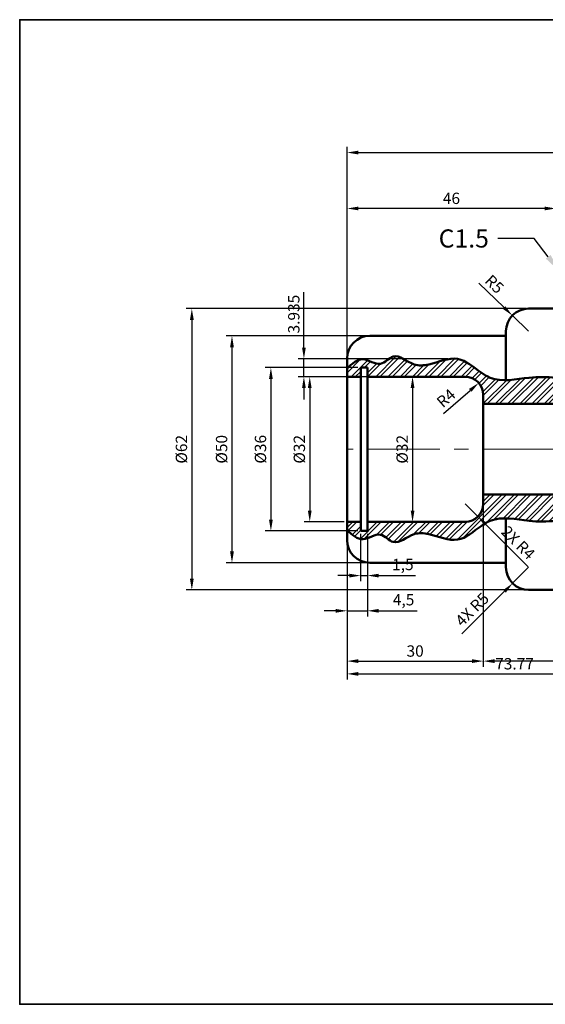
# Model space of a CAD drawing. Units: millimetres. Extents: x 14 to 362, y 30 to 247.
# Tile 1 of 3: x 14 to 130, y 30 to 247. Entities that reach past the tile are written whole.
import ezdxf
from ezdxf import colors
from ezdxf.entities.mleader import LeaderData, LeaderLine
from ezdxf.math import Vec2, Vec3

# ---------------------------------------------------------------- set-up
doc = ezdxf.new("R2010")
doc.units = ezdxf.units.MM
doc.header["$LTSCALE"] = 0.5
doc.linetypes.add('CENTER', pattern=[50.8, 31.75, -6.35, 6.35, -6.35])
for name, color, linetype, lineweight in [('M-CNTR', 1, 'CENTER', 18), ('M-DIMS', 2, 'Continuous', 25), ('M-HATC', 8, 'Continuous', 18), ('M-OUTL', 7, 'Continuous', 50), ('M-TTLB', 7, 'Continuous', 35)]:
    doc.layers.add(name, color=color, linetype=linetype, lineweight=lineweight)
doc.styles.get("Standard").update_dxf_attribs({"font": 'arial.ttf'})
doc.dimstyles.new('ISO-25', dxfattribs={"dimtxt": 2.5, "dimasz": 2.5, "dimexe": 1.25, "dimexo": 0.625, "dimtad": 1, "dimtxsty": 'Standard', "dimcen": 2.5, "dimadec": 0, "dimazin": 0, "dimtfac": 1, "dimtmove": 0, "dimatfit": 3, "dimfxl": 1, "dimarcsym": 0})

# ---------------------------------------------------------------- blocks, each defined once
blk = doc.blocks.new('*D1')
at = {"layer": 'Defpoints', "color": 0, "ltscale": 0.5, "transparency": 16777216}
for p in [(94.08, 177.22), (61.13, 127.22), (94.08, 127.22)]:
    blk.add_point(p, dxfattribs=at)
at = {"layer": 'M-DIMS', "color": 0, "lineweight": -2, "ltscale": 0.5, "transparency": 16777216}
for p, q in [((93.46, 177.22), (59.88, 177.22)), ((61.13, 174.72), (61.13, 129.72)), ((93.46, 127.22), (59.88, 127.22))]:
    blk.add_line(p, q, dxfattribs=at)
at = {"layer": 'M-DIMS', "color": 0, "ltscale": 0.5, "transparency": 16777216}
for points in [[(60.71, 174.72), (61.55, 174.72), (61.13, 177.22)], [(60.71, 129.72), (61.55, 129.72), (61.13, 127.22)]]:
    blk.add_solid(points, dxfattribs=at)
at = {"layer": 'M-DIMS', "color": 0, "ltscale": 0.5, "transparency": 16777216, "insert": (59.16, 152.22), "char_height": 2.5, "attachment_point": 5, "rotation": 90}
blk.add_mtext('%%C50', dxfattribs=at)
blk = doc.blocks.new('*D2')
at = {"layer": 'Defpoints', "color": 0, "ltscale": 0.5, "transparency": 16777216}
for p in [(89.47, 170.22), (69.7, 134.22), (89.47, 134.22)]:
    blk.add_point(p, dxfattribs=at)
at = {"layer": 'M-DIMS', "color": 0, "lineweight": -2, "ltscale": 0.5, "transparency": 16777216}
for p, q in [((88.85, 170.22), (68.45, 170.22)), ((69.7, 167.72), (69.7, 136.72)), ((88.85, 134.22), (68.45, 134.22))]:
    blk.add_line(p, q, dxfattribs=at)
at = {"layer": 'M-DIMS', "color": 0, "ltscale": 0.5, "transparency": 16777216}
for points in [[(69.28, 167.72), (70.12, 167.72), (69.7, 170.22)], [(69.28, 136.72), (70.12, 136.72), (69.7, 134.22)]]:
    blk.add_solid(points, dxfattribs=at)
at = {"layer": 'M-DIMS', "color": 0, "ltscale": 0.5, "transparency": 16777216, "insert": (67.73, 152.22), "char_height": 2.5, "attachment_point": 5, "rotation": 90}
blk.add_mtext('%%C36', dxfattribs=at)
blk = doc.blocks.new('*D3')
at = {"layer": 'Defpoints', "color": 0, "ltscale": 0.5, "transparency": 16777216}
for p in [(86.47, 168.22), (78.26, 136.22), (86.47, 136.22)]:
    blk.add_point(p, dxfattribs=at)
at = {"layer": 'M-DIMS', "color": 0, "lineweight": -2, "ltscale": 0.5, "transparency": 16777216}
for p, q in [((85.85, 168.22), (77.01, 168.22)), ((78.26, 165.72), (78.26, 138.72)), ((85.85, 136.22), (77.01, 136.22))]:
    blk.add_line(p, q, dxfattribs=at)
at = {"layer": 'M-DIMS', "color": 0, "ltscale": 0.5, "transparency": 16777216}
for points in [[(77.84, 165.72), (78.67, 165.72), (78.26, 168.22)], [(77.84, 138.72), (78.67, 138.72), (78.26, 136.22)]]:
    blk.add_solid(points, dxfattribs=at)
at = {"layer": 'M-DIMS', "color": 0, "ltscale": 0.5, "transparency": 16777216, "insert": (76.29, 152.22), "char_height": 2.5, "attachment_point": 5, "rotation": 90}
blk.add_mtext('%%C32', dxfattribs=at)
blk = doc.blocks.new('*D4')
at = {"layer": 'Defpoints', "color": 0, "ltscale": 0.5, "transparency": 16777216}
for p in [(126.47, 183.22), (52.29, 121.22), (126.47, 121.22)]:
    blk.add_point(p, dxfattribs=at)
at = {"layer": 'M-DIMS', "color": 0, "lineweight": -2, "ltscale": 0.5, "transparency": 16777216}
for p, q in [((125.85, 183.22), (51.04, 183.22)), ((52.29, 180.72), (52.29, 123.72)), ((125.85, 121.22), (51.04, 121.22))]:
    blk.add_line(p, q, dxfattribs=at)
at = {"layer": 'M-DIMS', "color": 0, "ltscale": 0.5, "transparency": 16777216}
for points in [[(51.87, 180.72), (52.71, 180.72), (52.29, 183.22)], [(51.87, 123.72), (52.71, 123.72), (52.29, 121.22)]]:
    blk.add_solid(points, dxfattribs=at)
at = {"layer": 'M-DIMS', "color": 0, "ltscale": 0.5, "transparency": 16777216, "insert": (50.32, 152.22), "char_height": 2.5, "attachment_point": 5, "rotation": 90}
blk.add_mtext('%%C62', dxfattribs=at)
blk = doc.blocks.new('*D5')
at = {"layer": 'Defpoints', "color": 0, "ltscale": 0.5, "transparency": 16777216}
for p in [(89.47, 134.22), (90.97, 134.22), (90.97, 124.38)]:
    blk.add_point(p, dxfattribs=at)
at = {"layer": 'M-DIMS', "color": 0, "lineweight": -2, "ltscale": 0.5, "transparency": 16777216}
for p, q in [((89.47, 133.6), (89.47, 123.13)), ((90.97, 133.6), (90.97, 123.13)), ((86.97, 124.38), (84.47, 124.38)), ((89.47, 124.38), (90.97, 124.38)), ((93.47, 124.38), (101.56, 124.38))]:
    blk.add_line(p, q, dxfattribs=at)
at = {"layer": 'M-DIMS', "color": 0, "ltscale": 0.5, "transparency": 16777216}
for points in [[(86.97, 124.79), (86.97, 123.96), (89.47, 124.38)], [(93.47, 124.79), (93.47, 123.96), (90.97, 124.38)]]:
    blk.add_solid(points, dxfattribs=at)
at = {"layer": 'M-DIMS', "color": 0, "ltscale": 0.5, "transparency": 16777216, "insert": (98.77, 126.5), "char_height": 2.5, "attachment_point": 5}
blk.add_mtext('1,5', dxfattribs=at)
blk = doc.blocks.new('*D6')
at = {"layer": 'Defpoints', "color": 0, "ltscale": 0.5, "transparency": 16777216}
for p in [(116.47, 142.22), (86.47, 132.22), (116.47, 105.53)]:
    blk.add_point(p, dxfattribs=at)
at = {"layer": 'M-DIMS', "color": 0, "lineweight": -2, "ltscale": 0.5, "transparency": 16777216}
for p, q in [((116.47, 141.6), (116.47, 104.28)), ((86.47, 131.6), (86.47, 104.28)), ((88.97, 105.53), (113.97, 105.53))]:
    blk.add_line(p, q, dxfattribs=at)
at = {"layer": 'M-DIMS', "color": 0, "ltscale": 0.5, "transparency": 16777216}
for points in [[(88.97, 105.95), (88.97, 105.11), (86.47, 105.53)], [(113.97, 105.95), (113.97, 105.11), (116.47, 105.53)]]:
    blk.add_solid(points, dxfattribs=at)
at = {"layer": 'M-DIMS', "color": 0, "ltscale": 0.5, "transparency": 16777216, "insert": (101.47, 107.43), "char_height": 2.5, "attachment_point": 5}
blk.add_mtext('30', dxfattribs=at)
blk = doc.blocks.new('*D7')
at = {"layer": 'Defpoints', "color": 0, "ltscale": 0.5, "transparency": 16777216}
for p in [(90.97, 125.68), (86.47, 117.94), (90.97, 116.62)]:
    blk.add_point(p, dxfattribs=at)
at = {"layer": 'M-DIMS', "color": 0, "lineweight": -2, "ltscale": 0.5, "transparency": 16777216}
for p, q in [((90.97, 125.06), (90.97, 115.37)), ((86.47, 117.31), (86.47, 115.37)), ((83.97, 116.62), (81.47, 116.62)), ((86.47, 116.62), (90.97, 116.62)), ((93.47, 116.62), (101.89, 116.62))]:
    blk.add_line(p, q, dxfattribs=at)
at = {"layer": 'M-DIMS', "color": 0, "ltscale": 0.5, "transparency": 16777216}
for points in [[(83.97, 117.03), (83.97, 116.2), (86.47, 116.62)], [(93.47, 117.03), (93.47, 116.2), (90.97, 116.62)]]:
    blk.add_solid(points, dxfattribs=at)
at = {"layer": 'M-DIMS', "color": 0, "ltscale": 0.5, "transparency": 16777216, "insert": (98.93, 118.74), "char_height": 2.5, "attachment_point": 5}
blk.add_mtext('4,5', dxfattribs=at)
blk = doc.blocks.new('*D8')
at = {"layer": 'Defpoints', "color": 0, "ltscale": 0.5, "transparency": 16777216}
for p in [(154.47, 142.22), (116.47, 115.92), (116.47, 105.53)]:
    blk.add_point(p, dxfattribs=at)
at = {"layer": 'M-DIMS', "color": 0, "lineweight": -2, "ltscale": 0.5, "transparency": 16777216}
for p, q in [((154.47, 141.6), (154.47, 104.28)), ((116.47, 115.3), (116.47, 104.28)), ((151.97, 105.53), (118.97, 105.53))]:
    blk.add_line(p, q, dxfattribs=at)
at = {"layer": 'M-DIMS', "color": 0, "ltscale": 0.5, "transparency": 16777216}
for points in [[(118.97, 105.95), (118.97, 105.11), (116.47, 105.53)], [(151.97, 105.95), (151.97, 105.11), (154.47, 105.53)]]:
    blk.add_solid(points, dxfattribs=at)
at = {"layer": 'M-DIMS', "color": 0, "ltscale": 0.5, "transparency": 16777216, "insert": (135.47, 107.43), "char_height": 2.5, "attachment_point": 5}
blk.add_mtext('38', dxfattribs=at)
blk = doc.blocks.new('*D11')
at = {"layer": 'Defpoints', "color": 0, "ltscale": 0.5, "transparency": 16777216}
for p in [(208.47, 217.62), (86.47, 172.22), (208.47, 152.22)]:
    blk.add_point(p, dxfattribs=at)
at = {"layer": 'M-DIMS', "color": 0, "lineweight": -2, "ltscale": 0.5, "transparency": 16777216}
for p, q in [((86.47, 172.85), (86.47, 218.87)), ((88.97, 217.62), (205.97, 217.62)), ((208.47, 152.85), (208.47, 218.87))]:
    blk.add_line(p, q, dxfattribs=at)
at = {"layer": 'M-DIMS', "color": 0, "ltscale": 0.5, "transparency": 16777216}
for points in [[(88.97, 218.04), (88.97, 217.2), (86.47, 217.62)], [(205.97, 218.04), (205.97, 217.2), (208.47, 217.62)]]:
    blk.add_solid(points, dxfattribs=at)
at = {"layer": 'M-DIMS', "color": 0, "ltscale": 0.5, "transparency": 16777216, "insert": (147.47, 219.5), "char_height": 2.5, "attachment_point": 5}
blk.add_mtext('122', dxfattribs=at)
blk = doc.blocks.new('*D12')
at = {"layer": 'Defpoints', "color": 0, "ltscale": 0.5, "transparency": 16777216}
for p in [(86.47, 205.29), (86.47, 190.72), (132.47, 190.72)]:
    blk.add_point(p, dxfattribs=at)
at = {"layer": 'M-DIMS', "color": 0, "lineweight": -2, "ltscale": 0.5, "transparency": 16777216}
for p, q in [((86.47, 191.35), (86.47, 206.54)), ((132.47, 191.35), (132.47, 206.54)), ((129.97, 205.29), (88.97, 205.29))]:
    blk.add_line(p, q, dxfattribs=at)
at = {"layer": 'M-DIMS', "color": 0, "ltscale": 0.5, "transparency": 16777216}
for points in [[(88.97, 205.71), (88.97, 204.88), (86.47, 205.29)], [(129.97, 205.71), (129.97, 204.88), (132.47, 205.29)]]:
    blk.add_solid(points, dxfattribs=at)
at = {"layer": 'M-DIMS', "color": 0, "ltscale": 0.5, "transparency": 16777216, "insert": (109.47, 207.2), "char_height": 2.5, "attachment_point": 5}
blk.add_mtext('46', dxfattribs=at)
blk = doc.blocks.new('*D24')
at = {"layer": 'Defpoints', "color": 0, "ltscale": 0.5, "transparency": 16777216}
for p in [(122.88, 181.7), (126.47, 178.22)]:
    blk.add_point(p, dxfattribs=at)
at = {"layer": 'M-DIMS', "color": 0, "lineweight": -2, "ltscale": 0.5, "transparency": 16777216}
for p, q in [((115.48, 188.86), (121.08, 183.44)), ((126.47, 178.22), (122.88, 181.7))]:
    blk.add_line(p, q, dxfattribs=at)
at = {"layer": 'M-DIMS', "color": 0, "ltscale": 0.5, "transparency": 16777216}
blk.add_solid([(121.37, 183.74), (120.8, 183.14), (122.88, 181.7)], dxfattribs=at)
at = {"layer": 'M-DIMS', "color": 0, "ltscale": 0.5, "transparency": 16777216, "insert": (118.7, 188.38), "char_height": 2.5, "attachment_point": 5, "rotation": 315.9281}
blk.add_mtext('R5', dxfattribs=at)
blk = doc.blocks.new('*D25')
at = {"layer": 'Defpoints', "color": 0, "ltscale": 0.5, "transparency": 16777216}
for p in [(115.49, 166.85), (112.47, 164.22)]:
    blk.add_point(p, dxfattribs=at)
at = {"layer": 'M-DIMS', "color": 0, "lineweight": -2, "ltscale": 0.5, "transparency": 16777216}
blk.add_line((107.74, 160.1), (113.6, 165.21), dxfattribs=at)
at = {"layer": 'M-DIMS', "color": 0, "ltscale": 0.5, "transparency": 16777216}
blk.add_solid([(113.33, 165.52), (113.88, 164.89), (115.49, 166.85)], dxfattribs=at)
at = {"layer": 'M-DIMS', "color": 0, "ltscale": 0.5, "transparency": 16777216, "insert": (108.5, 163.25), "char_height": 2.5, "attachment_point": 5, "rotation": 41.0414}
blk.add_mtext('R4', dxfattribs=at)
blk = doc.blocks.new('*D27')
at = {"layer": 'Defpoints', "color": 0, "ltscale": 0.5, "transparency": 16777216}
for p in [(101.72, 168.22), (100.9, 136.22), (101.72, 136.22)]:
    blk.add_point(p, dxfattribs=at)
at = {"layer": 'M-DIMS', "color": 0, "lineweight": -2, "ltscale": 0.5, "transparency": 16777216}
for p, q in [((101.1, 168.22), (99.65, 168.22)), ((100.9, 165.72), (100.9, 138.72)), ((101.1, 136.22), (99.65, 136.22))]:
    blk.add_line(p, q, dxfattribs=at)
at = {"layer": 'M-DIMS', "color": 0, "ltscale": 0.5, "transparency": 16777216}
for points in [[(100.49, 165.72), (101.32, 165.72), (100.9, 168.22)], [(100.49, 138.72), (101.32, 138.72), (100.9, 136.22)]]:
    blk.add_solid(points, dxfattribs=at)
at = {"layer": 'M-DIMS', "color": 0, "ltscale": 0.5, "transparency": 16777216, "insert": (98.93, 152.22), "char_height": 2.5, "attachment_point": 5, "rotation": 90}
blk.add_mtext('%%C32', dxfattribs=at)
blk = doc.blocks.new('*D29')
at = {"layer": 'Defpoints', "color": 0, "ltscale": 0.5, "transparency": 16777216}
for p in [(160.25, 152.22), (86.47, 136.22), (160.25, 102.72)]:
    blk.add_point(p, dxfattribs=at)
at = {"layer": 'M-DIMS', "color": 0, "lineweight": -2, "ltscale": 0.5, "transparency": 16777216}
for p, q in [((160.25, 151.6), (160.25, 101.47)), ((86.47, 135.6), (86.47, 101.47)), ((88.97, 102.72), (157.75, 102.72))]:
    blk.add_line(p, q, dxfattribs=at)
at = {"layer": 'M-DIMS', "color": 0, "ltscale": 0.5, "transparency": 16777216}
for points in [[(88.97, 103.14), (88.97, 102.3), (86.47, 102.72)], [(157.75, 103.14), (157.75, 102.3), (160.25, 102.72)]]:
    blk.add_solid(points, dxfattribs=at)
at = {"layer": 'M-DIMS', "color": 0, "ltscale": 0.5, "transparency": 16777216, "insert": (123.36, 104.62), "char_height": 2.5, "attachment_point": 5}
blk.add_mtext('73.77', dxfattribs=at)
blk = doc.blocks.new('*D30')
at = {"layer": 'Defpoints', "color": 0, "ltscale": 0.5, "transparency": 16777216}
for p in [(76.97, 172.15), (109.31, 172.15), (112.47, 168.22)]:
    blk.add_point(p, dxfattribs=at)
at = {"layer": 'M-DIMS', "color": 0, "lineweight": -2, "ltscale": 0.5, "transparency": 16777216}
for p, q in [((76.97, 174.65), (76.97, 186.86)), ((108.68, 172.15), (75.72, 172.15)), ((76.97, 168.22), (76.97, 172.15)), ((111.85, 168.22), (75.72, 168.22)), ((76.97, 165.72), (76.97, 163.22))]:
    blk.add_line(p, q, dxfattribs=at)
at = {"layer": 'M-DIMS', "color": 0, "ltscale": 0.5, "transparency": 16777216}
for points in [[(76.56, 174.65), (77.39, 174.65), (76.97, 172.15)], [(76.56, 165.72), (77.39, 165.72), (76.97, 168.22)]]:
    blk.add_solid(points, dxfattribs=at)
at = {"layer": 'M-DIMS', "color": 0, "ltscale": 0.5, "transparency": 16777216, "insert": (75.07, 182.01), "char_height": 2.5, "attachment_point": 5, "rotation": 90}
blk.add_mtext('3.935', dxfattribs=at)
blk = doc.blocks.new('*D33')
at = {"layer": 'Defpoints', "color": 0, "ltscale": 0.5, "transparency": 16777216}
for p in [(126.47, 126.22), (122.94, 122.68)]:
    blk.add_point(p, dxfattribs=at)
at = {"layer": 'M-DIMS', "color": 0, "lineweight": -2, "ltscale": 0.5, "transparency": 16777216}
for p, q in [((126.47, 126.22), (122.94, 122.68)), ((111.78, 111.53), (121.17, 120.92))]:
    blk.add_line(p, q, dxfattribs=at)
at = {"layer": 'M-DIMS', "color": 0, "ltscale": 0.5, "transparency": 16777216}
blk.add_solid([(120.88, 121.21), (121.46, 120.62), (122.94, 122.68)], dxfattribs=at)
at = {"layer": 'M-DIMS', "color": 0, "ltscale": 0.5, "transparency": 16777216, "insert": (114.25, 116.68), "char_height": 2.5, "attachment_point": 5, "rotation": 44.9981}
blk.add_mtext('4X R5', dxfattribs=at)
blk = doc.blocks.new('*D34')
at = {"layer": 'Defpoints', "color": 0, "ltscale": 0.5, "transparency": 16777216}
for p in [(112.47, 140.22), (115.3, 137.39)]:
    blk.add_point(p, dxfattribs=at)
at = {"layer": 'M-DIMS', "color": 0, "lineweight": -2, "ltscale": 0.5, "transparency": 16777216}
for p, q in [((112.47, 140.22), (115.3, 137.39)), ((126.39, 126.3), (117.07, 135.62))]:
    blk.add_line(p, q, dxfattribs=at)
at = {"layer": 'M-DIMS', "color": 0, "ltscale": 0.5, "transparency": 16777216}
blk.add_solid([(117.36, 135.92), (116.78, 135.33), (115.3, 137.39)], dxfattribs=at)
at = {"layer": 'M-DIMS', "color": 0, "ltscale": 0.5, "transparency": 16777216, "insert": (123.95, 131.41), "char_height": 2.5, "attachment_point": 5, "rotation": 315.0057}
blk.add_mtext('2X R4', dxfattribs=at)

msp = doc.modelspace()

# ---------------------------------------------------------------- hatches: boundary and pattern name
at = {"layer": 'M-HATC', "ltscale": 0.5}
h = msp.add_hatch(dxfattribs=at)
h.set_pattern_fill('ANSI32', color=256, scale=0.2)
edge = h.paths.add_edge_path()
edge.add_spline(control_points=[(155.9733, 166.9662), (154.0211, 166.7606), (152.3026, 167.0826), (150.4948, 166.9658), (150.4733, 166.9643)], knot_values=[66.79219469, 66.79219469, 66.79219469, 66.79219469, 72.22935864, 72.29469704, 72.29469704, 72.29469704, 72.29469704], degree=3, periodic=0)
edge.add_spline(control_points=[(150.4733, 166.9643), (148.1871, 166.8102), (145.7606, 165.9737), (143.4733, 166.4419)], knot_values=[59.83740681, 59.83740681, 59.83740681, 59.83740681, 66.79219469, 66.79219469, 66.79219469, 66.79219469], degree=3, periodic=0)
edge.add_spline(control_points=[(143.4733, 166.4419), (142.9655, 166.5458), (142.4644, 166.7141), (141.9733, 166.9685)], knot_values=[58.29313338, 58.29313338, 58.29313338, 58.29313338, 59.83740681, 59.83740681, 59.83740681, 59.83740681], degree=3, periodic=0)
edge.add_spline(control_points=[(141.9733, 166.9685), (140.9547, 167.424), (139.4266, 168.1074), (136.6788, 167.9381), (135.0539, 167.967), (133.9733, 167.9862)], knot_values=[50.13092632, 50.13092632, 50.13092632, 50.13092632, 53.40454911, 55.04224579, 58.29313338, 58.29313338, 58.29313338, 58.29313338], degree=3, periodic=0)
edge.add_spline(control_points=[(133.9733, 167.9862), (133.4945, 167.87), (132.981, 167.9345), (132.4733, 167.9862)], knot_values=[48.63092632, 48.63092632, 48.63092632, 48.63092632, 50.13092632, 50.13092632, 50.13092632, 50.13092632], degree=3, periodic=0)
edge.add_spline(control_points=[(132.4733, 167.9862), (130.4688, 168.1902), (126.9587, 168.1975), (123.1381, 167.4912), (121.4733, 167.4533)], knot_values=[37.76376912, 37.76376912, 37.76376912, 37.76376912, 43.68697215, 48.63092632, 48.63092632, 48.63092632, 48.63092632], degree=3, periodic=0)
edge.add_spline(control_points=[(121.4733, 167.4533), (120.2624, 167.4257), (118.3251, 167.6279), (114.9522, 169.7579), (110.8651, 173.4299), (105.5597, 170.8967), (100.6595, 170.4149), (97.032, 174.1091), (93.7472, 169.8507), (89.8165, 173.1693), (87.5914, 171.0802), (86.4733, 170.0306)], knot_values=[0, 0, 0, 0, 3.59607393, 5.94391752, 11.88748547, 18.33997532, 21.58498162, 26.51526036, 29.7147102, 33.71957019, 37.76376912, 37.76376912, 37.76376912, 37.76376912], degree=3, periodic=0)
edge.add_line((86.4733, 170.0306), (86.4733, 168.2201))
edge.add_line((86.4733, 168.2201), (89.4733, 168.2201))
edge.add_line((89.4733, 168.2201), (89.4733, 170.2201))
edge.add_line((89.4733, 170.2201), (90.9733, 170.2201))
edge.add_line((90.9733, 170.2201), (90.9733, 168.2201))
edge.add_line((90.9733, 168.2201), (112.4733, 168.2201))
edge.add_arc((112.4733, 164.2201), 4, 0, 90, ccw=False)
edge.add_line((116.4733, 164.2201), (116.4733, 162.2201))
edge.add_line((116.4733, 162.2201), (154.4733, 162.2201))
edge.add_line((154.4733, 162.2201), (155.9733, 159.622))
edge.add_line((155.9733, 159.622), (155.9733, 166.9662))
edge = h.paths.add_edge_path()
edge.add_spline(control_points=[(165.9849, 152.2201), (166.1094, 154.2843), (166.0108, 157.4665), (163.8675, 160.5177), (162.4341, 162.7097), (161.6725, 164.7478), (161.4733, 165.2055)], knot_values=[78.81028285, 78.81028285, 78.81028285, 78.81028285, 83.42605774, 85.79814935, 90.2231733, 91.61225648, 91.61225648, 91.61225648, 91.61225648], degree=3, periodic=0)
edge.add_spline(control_points=[(161.4733, 165.2055), (161.1482, 165.953), (160.0862, 167.8712), (157.5064, 167.129), (155.9806, 166.9669), (155.9733, 166.9662)], knot_values=[72.29469704, 72.29469704, 72.29469704, 72.29469704, 74.5626758, 78.79015553, 78.81028285, 78.81028285, 78.81028285, 78.81028285], degree=3, periodic=0)
edge.add_line((155.9733, 166.9662), (155.9733, 159.622))
edge.add_line((155.9733, 159.622), (160.2468, 152.2201))
edge.add_line((160.2468, 152.2201), (165.9849, 152.2201))
edge = h.paths.add_edge_path()
edge.add_spline(control_points=[(161.4733, 139.2347), (161.6725, 139.6924), (162.4341, 141.7305), (163.8675, 143.9225), (166.0108, 146.9737), (166.1094, 150.1559), (165.9849, 152.2201)], knot_values=[78.81028285, 78.81028285, 78.81028285, 78.81028285, 80.19936602, 84.62438998, 86.99648158, 91.61225648, 91.61225648, 91.61225648, 91.61225648], degree=3, periodic=0)
edge.add_line((165.9849, 152.2201), (160.2468, 152.2201))
edge.add_line((160.2468, 152.2201), (155.9733, 144.8182))
edge.add_line((155.9733, 144.8182), (155.9733, 137.474))
edge.add_spline(control_points=[(155.9733, 137.474), (155.9806, 137.4733), (157.5064, 137.3112), (160.0862, 136.569), (161.1482, 138.4872), (161.4733, 139.2347)], knot_values=[72.29469704, 72.29469704, 72.29469704, 72.29469704, 72.31482436, 76.54230409, 78.81028285, 78.81028285, 78.81028285, 78.81028285], degree=3, periodic=0)
edge = h.paths.add_edge_path()
edge.add_line((155.9733, 144.8182), (154.4733, 142.2201))
edge.add_line((154.4733, 142.2201), (116.4733, 142.2201))
edge.add_line((116.4733, 142.2201), (116.4733, 140.2201))
edge.add_arc((112.4733, 140.2201), 4, -90, 0, ccw=False)
edge.add_line((112.4733, 136.2201), (90.9733, 136.2201))
edge.add_line((90.9733, 136.2201), (90.9733, 134.2201))
edge.add_line((90.9733, 134.2201), (89.4733, 134.2201))
edge.add_line((89.4733, 134.2201), (89.4733, 136.2201))
edge.add_line((89.4733, 136.2201), (86.4733, 136.2201))
edge.add_line((86.4733, 136.2201), (86.4733, 134.4096))
edge.add_spline(control_points=[(86.4733, 134.4096), (87.5914, 133.36), (89.8165, 131.2709), (93.7472, 134.5895), (97.032, 130.3311), (100.6595, 134.0253), (105.5597, 133.5435), (110.8651, 131.0103), (114.9522, 134.6823), (118.3251, 136.8123), (120.2624, 137.0145), (121.4733, 136.9869)], knot_values=[0, 0, 0, 0, 4.04419892, 8.04905892, 11.24850875, 16.1787875, 19.42379379, 25.87628365, 31.81985159, 34.16769518, 37.76376912, 37.76376912, 37.76376912, 37.76376912], degree=3, periodic=0)
edge.add_spline(control_points=[(121.4733, 136.9869), (123.1381, 136.949), (126.9587, 136.2427), (130.4688, 136.25), (132.4733, 136.454)], knot_values=[37.76376912, 37.76376912, 37.76376912, 37.76376912, 42.70772329, 48.63092632, 48.63092632, 48.63092632, 48.63092632], degree=3, periodic=0)
edge.add_spline(control_points=[(132.4733, 136.454), (132.981, 136.5057), (133.4945, 136.5702), (133.9733, 136.454)], knot_values=[48.63092632, 48.63092632, 48.63092632, 48.63092632, 50.13092632, 50.13092632, 50.13092632, 50.13092632], degree=3, periodic=0)
edge.add_spline(control_points=[(133.9733, 136.454), (135.0539, 136.4733), (136.6788, 136.5021), (139.4266, 136.3328), (140.9547, 137.0162), (141.9733, 137.4717)], knot_values=[50.13092632, 50.13092632, 50.13092632, 50.13092632, 53.38181392, 55.0195106, 58.29313338, 58.29313338, 58.29313338, 58.29313338], degree=3, periodic=0)
edge.add_spline(control_points=[(141.9733, 137.4717), (142.4644, 137.7261), (142.9655, 137.8944), (143.4733, 137.9983)], knot_values=[58.29313338, 58.29313338, 58.29313338, 58.29313338, 59.83740681, 59.83740681, 59.83740681, 59.83740681], degree=3, periodic=0)
edge.add_spline(control_points=[(143.4733, 137.9983), (145.7606, 138.4665), (148.1871, 137.63), (150.4733, 137.4759)], knot_values=[59.83740681, 59.83740681, 59.83740681, 59.83740681, 66.79219469, 66.79219469, 66.79219469, 66.79219469], degree=3, periodic=0)
edge.add_spline(control_points=[(150.4733, 137.4759), (150.4948, 137.4744), (152.3026, 137.3576), (154.0211, 137.6796), (155.9733, 137.474)], knot_values=[66.79219469, 66.79219469, 66.79219469, 66.79219469, 66.85753309, 72.29469704, 72.29469704, 72.29469704, 72.29469704], degree=3, periodic=0)
edge.add_line((155.9733, 137.474), (155.9733, 144.8182))

# ---------------------------------------------------------------- linework, layer by layer
at = {"layer": 'M-CNTR'}
msp.add_line((208.4733, 152.2201), (86.4733, 152.2201), dxfattribs=at)
at = {"layer": 'M-OUTL'}
for p, q in [((126.4733, 183.2201), (132.4733, 183.2201)), ((121.4733, 178.2201), (121.4733, 167.4533)), ((91.4733, 177.2201), (121.4733, 177.2201)), ((86.4733, 172.2201), (86.4733, 132.2201)), ((89.4733, 170.2201), (89.4733, 134.2201)), ((90.9733, 170.2201), (89.4733, 170.2201)), ((90.9733, 134.2201), (90.9733, 170.2201)), ((86.4733, 168.2201), (89.4733, 168.2201)), ((90.9733, 168.2201), (112.4733, 168.2201)), ((116.4733, 164.2201), (116.4733, 140.2201)), ((116.4733, 162.2201), (154.4733, 162.2201)), ((154.4733, 142.2201), (116.4733, 142.2201)), ((121.4733, 136.9869), (121.4733, 126.2201)), ((89.4733, 136.2201), (86.4733, 136.2201)), ((112.4733, 136.2201), (90.9733, 136.2201)), ((89.4733, 134.2201), (90.9733, 134.2201)), ((121.4733, 127.2201), (91.4733, 127.2201)), ((126.4733, 121.2201), (132.4733, 121.2201))]:
    msp.add_line(p, q, dxfattribs=at)
for centre, radius, start, end in [((126.4733, 178.2201), 5, 90, 180), ((91.4733, 172.2201), 5, 90, 180), ((112.4733, 164.2201), 4, 0, 90), ((112.4733, 140.2201), 4, 270, 0), ((91.4733, 132.2201), 5, 180, 270), ((126.4733, 126.2201), 5, 180, 270)]:
    msp.add_arc(centre, radius, start, end, dxfattribs=at)
for points in [[(86.4733, 170.0306), (87.5914, 171.0802), (89.8165, 173.1693), (93.7472, 169.8507), (97.032, 174.1091), (100.6595, 170.4149), (105.5597, 170.8967), (110.8651, 173.4299), (114.9522, 169.7579), (119.7279, 166.742), (125.7971, 168.1999), (130.9533, 168.1892), (133.4945, 167.87), (133.9733, 167.9862), (135.0539, 167.967), (136.6788, 167.9381), (139.4266, 168.1074), (140.9547, 167.424), (141.9733, 166.9685), (144.6969, 165.5578), (149.6555, 167.5829), (155.3537, 166.5097), (160.6362, 168.0294), (162.037, 163.317), (163.8675, 160.5177), (166.0108, 157.4665), (166.1094, 154.2843), (165.9849, 152.2201)], [(86.4733, 134.4096), (87.5914, 133.36), (89.8165, 131.2709), (93.7472, 134.5895), (97.032, 130.3311), (100.6595, 134.0253), (105.5597, 133.5435), (110.8651, 131.0103), (114.9522, 134.6823), (119.7279, 137.6982), (125.7971, 136.2403), (130.9533, 136.251), (133.4945, 136.5702), (133.9733, 136.454), (135.0539, 136.4733), (136.6788, 136.5021), (139.4266, 136.3328), (140.9547, 137.0162), (141.9733, 137.4717), (144.6969, 138.8824), (149.6555, 136.8573), (155.3537, 137.9305), (160.6362, 136.4108), (162.037, 141.1233), (163.8675, 143.9225), (166.0108, 146.9737), (166.1094, 150.1559), (165.9849, 152.2201)]]:
    msp.add_open_spline(points, degree=3, knots=[0, 0, 0, 0, 4.04419892, 8.04905892, 11.24850875, 16.1787875, 19.42379379, 25.87628365, 31.81985159, 34.16769518, 42.70772329, 48.63092632, 50.13092632, 50.13092632, 50.13092632, 53.38181392, 55.0195106, 58.29313338, 58.29313338, 58.29313338, 66.85753309, 72.31482436, 76.54230409, 80.19936602, 84.62438998, 86.99648158, 91.61225648, 91.61225648, 91.61225648, 91.61225648], dxfattribs=at)
at = {"layer": 'M-TTLB', "ltscale": 0.5}
msp.add_lwpolyline([(361.563, 29.8922), (14.3774, 29.8922), (14.3774, 246.8988), (361.563, 246.8988)], close=True, dxfattribs=at)

# ---------------------------------------------------------------- dimensions: what is measured, and where the dimension line sits
at = {"layer": 'M-DIMS', "ltscale": 0.5}
for base, p1, p2, override, picture, middle in [((208.4733, 217.6202), (86.4733, 172.2201), (208.4733, 152.2201), {"dimclrd": 0, "dimclre": 0, "dimclrt": 0}, '*D11', (147.4733, 219.5004)), ((86.4733, 205.2939), (132.4733, 190.7201), (86.4733, 190.7201), {"dimclrd": 0, "dimclre": 0, "dimclrt": 0}, '*D12', (109.4733, 207.1953)), ((160.2468, 102.7201), (86.4733, 136.2201), (160.2468, 152.2201), {"dimdec": 2, "dimlfac": 1, "dimrnd": 0, "dimzin": 0, "dimdsep": 46, "dimlunit": 2}, '*D29', (123.3601, 104.6224)), ((116.4733, 105.5312), (86.4733, 132.2201), (116.4733, 142.2201), {"dimclrd": 0, "dimclre": 0, "dimclrt": 0}, '*D6', (101.4733, 107.4335)), ((116.4733, 105.5312), (154.4733, 142.2201), (116.4733, 115.9221), {"dimclrd": 0, "dimclre": 0, "dimclrt": 0}, '*D8', (135.4733, 107.4335)), ((90.9733, 124.377), (89.4733, 134.2201), (90.9733, 134.2201), {"dimclrd": 0, "dimclre": 0, "dimclrt": 0}, '*D5', (98.7658, 126.5043)), ((90.9733, 116.6182), (86.4733, 117.9382), (90.9733, 125.6831), {"dimclrd": 0, "dimclre": 0, "dimclrt": 0}, '*D7', (98.9338, 118.7404))]:
    dim = msp.add_linear_dim(base=base, p1=p1, p2=p2, dimstyle='ISO-25', override=override, dxfattribs=at)
    dim.commit()
    dim.dimension.update_dxf_attribs({"geometry": picture, "text_midpoint": middle})
dim = msp.add_radius_dim(center=(126.4733, 178.2201), mpoint=(122.881, 181.6979), dimstyle='ISO-25', override={"dimclrd": 0, "dimclre": 0, "dimclrt": 0}, dxfattribs=at)
dim.commit()
dim.dimension.update_dxf_attribs({"geometry": '*D24', "text_midpoint": (118.7037, 188.3814)})
dim = msp.add_linear_dim(base=(76.9733, 172.1548), p1=(112.4733, 168.2201), p2=(109.3087, 172.1548), angle=90, dimstyle='ISO-25', override={"dimdec": 3, "dimlfac": 1, "dimrnd": 0, "dimzin": 0, "dimdsep": 46, "dimlunit": 2}, dxfattribs=at)
dim.commit()
dim.dimension.update_dxf_attribs({"geometry": '*D30', "text_midpoint": (75.0711, 182.0065)})
for base, p1, p2, picture, middle in [((52.2889, 121.2201), (126.4733, 183.2201), (126.4733, 121.2201), '*D4', (50.3176, 152.2201)), ((61.1293, 127.2201), (94.0819, 177.2201), (94.0819, 127.2201), '*D1', (59.1579, 152.2201)), ((69.7016, 134.2201), (89.4733, 170.2201), (89.4733, 134.2201), '*D2', (67.7302, 152.2201)), ((78.2579, 136.2201), (86.4733, 168.2201), (86.4733, 136.2201), '*D3', (76.2866, 152.2201)), ((100.9035, 136.2201), (101.7233, 168.2201), (101.7233, 136.2201), '*D27', (98.9321, 152.2201))]:
    dim = msp.add_linear_dim(base=base, p1=p1, p2=p2, angle=90, text='%%C<>', dimstyle='ISO-25', override={"dimclrd": 0, "dimclre": 0, "dimclrt": 0}, dxfattribs=at)
    dim.commit()
    dim.dimension.update_dxf_attribs({"geometry": picture, "text_midpoint": middle})
dim = msp.add_radius_dim(center=(112.4733, 164.2201), mpoint=(115.4903, 166.8465), dimstyle='ISO-25', override={"dimclrd": 0, "dimclre": 0, "dimclrt": 0}, dxfattribs=at)
dim.commit()
dim.dimension.update_dxf_attribs({"geometry": '*D25', "text_midpoint": (109.7313, 161.833), "dimtype": 164})
for center, mpoint, text, picture, middle in [((112.4733, 140.2201), (115.302, 137.392), '2X <>', '*D34', (123.9461, 131.4094)), ((126.4733, 126.2201), (122.9377, 122.6847), '4X <>', '*D33', (114.2524, 116.6817))]:
    dim = msp.add_radius_dim(center=center, mpoint=mpoint, text=text, dimstyle='ISO-25', override={"dimdec": 0, "dimlfac": 1, "dimrnd": 0, "dimzin": 0, "dimdsep": 46, "dimlunit": 2}, dxfattribs=at)
    dim.commit()
    dim.dimension.update_dxf_attribs({"geometry": picture, "text_midpoint": middle})

# ---------------------------------------------------------------- leaders
ml = msp.add_multileader_mtext('Standard', dxfattribs=at)
ml.set_content('C1.5', color=256)
ml.set_leader_properties()
ml.build(insert=Vec2(0, 0))
ctx = ml.context
ctx.base_point, ctx.plane_origin = Vec3(104.4086, 198.6455), Vec3(133.2233, 191.4701)
ctx.text_align_type = 2
notes = []
notes.append((ctx, [(0, (1, 1, 0), (127.7101, 198.6455), (-1, 0), 8, [(0, [(133.2233, 191.4701)], 0, [])])]))
ctx.mtext.insert, ctx.mtext.alignment, ctx.mtext.flow_direction = Vec3(117.7101, 200.6796), 3, 5
for ctx, leaders in notes:
    for number, flags, end, landing, length, lines in leaders:
        leader = LeaderData()
        leader.index, (leader.has_last_leader_line, leader.has_dogleg_vector, leader.attachment_direction) = number, flags
        leader.last_leader_point, leader.dogleg_vector, leader.dogleg_length = Vec3(end), Vec3(landing), length
        for number, points, colour, breaks in lines:
            line = LeaderLine()
            line.index, line.vertices, line.color, line.breaks = number, Vec3.list(points), colors.encode_raw_color(colour), breaks
            leader.lines.append(line)
        ctx.leaders.append(leader)

doc.saveas('drawing.dxf')
